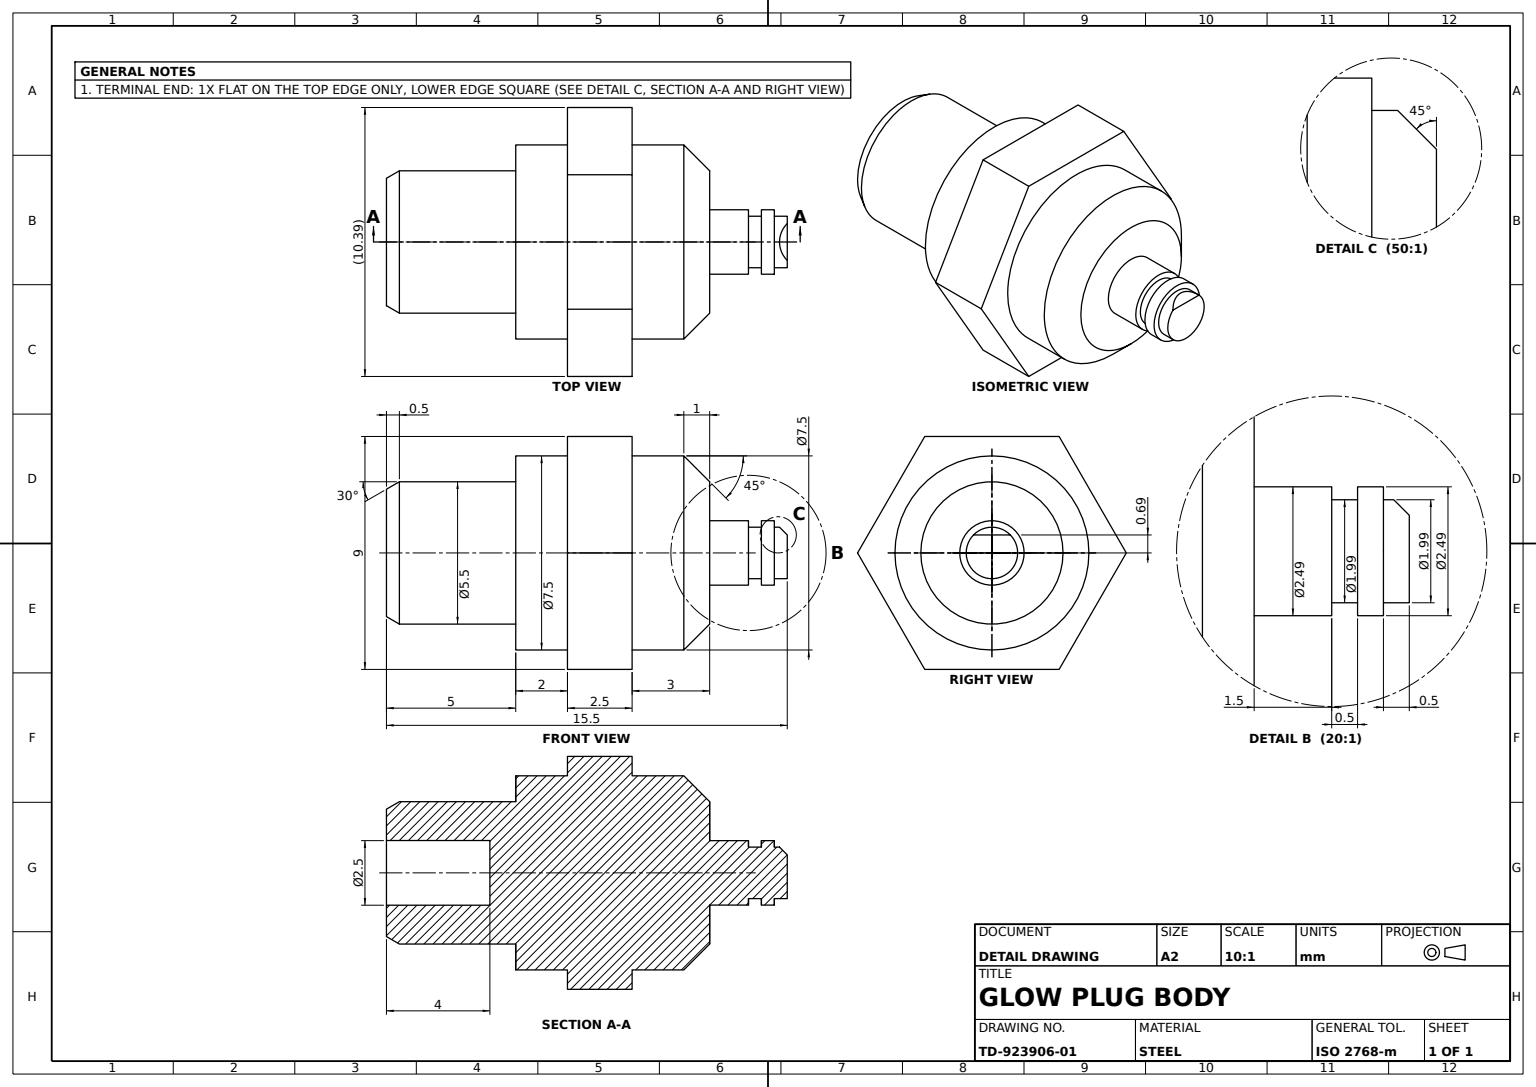
from build123d import *

# Parameters (mm, degrees)
HEX_BODY_9AF_DEPTH            = 2.5
COLLAR_7_5_SKETCH_R           = 3.75
COLLAR_7_5_DEPTH              = 2
TIP_BODY_5_5_SKETCH_R         = 2.75
TIP_BODY_5_5_DEPTH            = 5
TIP_END_CHAMFER_0_5X30_SIZE   = 0.5
TIP_END_CHAMFER_0_5X30_SIZE2  = 0.288675135
TIP_BORE_2_5_SKETCH_R         = 1.25
TIP_BORE_2_5_DEPTH            = 4
SHANK_START                   = 3
SHANK_7_5_SKETCH_R            = 3.75
SHANK_7_5_DEPTH               = 3
SHANK_CHAMFER_1X45_SIZE       = 1
TERMINAL_NOTCH_CUT_DEPTH      = 12.7260394
TERMINAL_NOTCH_CUT_DEPTH_BACK = 12.7260394


with BuildPart() as part:
    # Hex Profile 9AF Sketch → Hex Body 9AF (new body)
    with BuildSketch(Plane.XY):
        Polygon((2.598076211, 4.5), (-2.598076211, 4.5), (-5.196152423, 0), (-2.598076211, -4.5), (2.598076211, -4.5), (5.196152423, 0), align=None)
    extrude(amount=HEX_BODY_9AF_DEPTH)

    # Collar Ø7.5 Sketch → Collar Ø7.5 (add)
    with BuildSketch(Plane.XY.offset(2.5)):
        Circle(COLLAR_7_5_SKETCH_R)
    extrude(amount=COLLAR_7_5_DEPTH)

    # Tip Body Ø5.5 Sketch → Tip Body Ø5.5 (add)
    with BuildSketch(Plane.XY.offset(4.5)):
        Circle(TIP_BODY_5_5_SKETCH_R)
    extrude(amount=TIP_BODY_5_5_DEPTH)

    # Tip End Chamfer 0.5x30
    tip_end_chamfer_0_5x30_edges = [part.edges().sort_by_distance(p)[0] for p in [
        (-2.75, 0, 9.5),
    ]]
    tip_end_chamfer_0_5x30_side = [part.faces().sort_by_distance(p)[0] for p in [
        (-2.75, 0, 7),
    ]]
    chamfer(tip_end_chamfer_0_5x30_edges, length=TIP_END_CHAMFER_0_5X30_SIZE, length2=TIP_END_CHAMFER_0_5X30_SIZE2, reference=tip_end_chamfer_0_5x30_side[0])

    # Tip Bore Ø2.5 Sketch → Tip Bore Ø2.5 (cut)
    with BuildSketch(Plane.XY.offset(9.5)):
        Circle(TIP_BORE_2_5_SKETCH_R)
    extrude(amount=-TIP_BORE_2_5_DEPTH, mode=Mode.SUBTRACT)

    # Shank Ø7.5 Sketch → Shank Ø7.5 (add)
    with BuildSketch(Plane(origin=(0, 0, 0), x_dir=(-1, 0, 0), z_dir=(0, 0, -1)).offset(SHANK_START)):
        with Locations(Location((0, 0, 0), (0, 0, 180))):
            Circle(SHANK_7_5_SKETCH_R)
    extrude(amount=-SHANK_7_5_DEPTH)

    # Shank Chamfer 1x45
    shank_chamfer_1x45_edges = [part.edges().sort_by_distance(p)[0] for p in [
        (-3.75, 0, -3),
    ]]
    chamfer(shank_chamfer_1x45_edges, length=SHANK_CHAMFER_1X45_SIZE)

    # Terminal Stud Profile Sketch → Terminal Stud (revolve)
    with BuildSketch(Plane(origin=(0, 0, 0), x_dir=(0, 0, -1), z_dir=(1, 0, 0)), mode=Mode.PRIVATE) as terminal_stud_sk:
        Polygon((3, -1.245), (4.5, -1.245), (4.5, -0.995), (5, -0.995), (5, -1.245), (5.5, -1.245), (5.5, -0.995), (6, -0.995), (6, 0), (3, 0), align=None)
    revolve(terminal_stud_sk.sketch.rotate(Axis((0, 0, -3), (0, 0, -1)), 270), axis=Axis((0, 0, -3), (0, 0, -1)))

    # Terminal Notch Sketch → Terminal Notch Cut (cut, two sides: drawn at the far end of the back side and taken through both)
    with BuildSketch(Plane(origin=(0, 0, 0), x_dir=(0, 0, -1), z_dir=(1, 0, 0)).offset(-TERMINAL_NOTCH_CUT_DEPTH_BACK)):
        Polygon((6, 0.695), (5.7, 0.995), (6, 0.995), align=None)
    extrude(amount=TERMINAL_NOTCH_CUT_DEPTH + TERMINAL_NOTCH_CUT_DEPTH_BACK, mode=Mode.SUBTRACT)


solid = part.part
